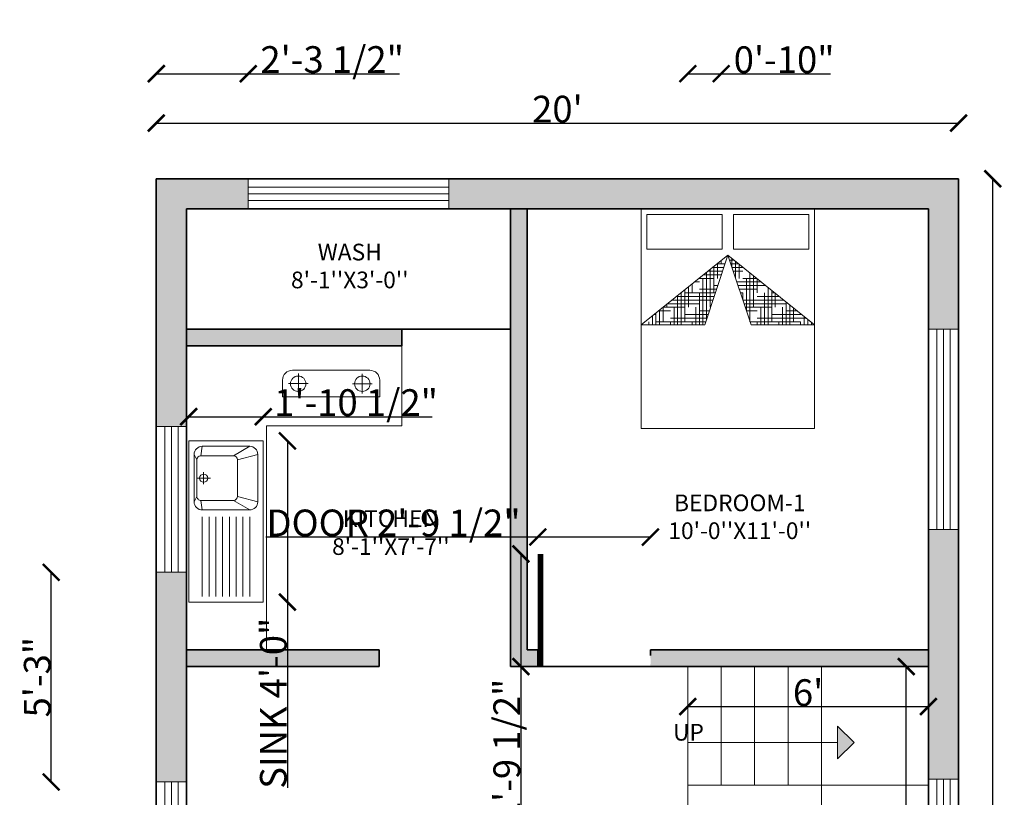
# Model space of a CAD drawing. Units: inches. Extents: x 2267 to 2908, y 1531 to 2136.
# Tile 3 of 5: x 2267 to 2562, y 1882 to 2115. Entities that reach past the tile are written whole.
import ezdxf

# ---------------------------------------------------------------- set-up
doc = ezdxf.new("R2010")
doc.units = ezdxf.units.IN
for name, color, linetype, lineweight in [('A-ANNO-DIMS', 2, 'Continuous', 18), ('A-ANNO-SYMB', 50, 'Continuous', 18), ('A-ANNO-TEXT', 7, 'Continuous', 18), ('A-AREA-IDEN', 7, 'Continuous', 18), ('A-EQPM', 9, 'Continuous', 18), ('A-FLOR-FIXT', 9, 'Continuous', 18), ('A-FURN', 9, 'Continuous', 18), ('A-WALL-PATT', 8, 'Continuous', 13), ('DOOR', 30, 'Continuous', 18), ('KITCHEN', 80, 'Continuous', 18), ('STEPS', 50, 'Continuous', 18), ('WALL', 7, 'Continuous', 35), ('WINDOW', 152, 'Continuous', 18)]:
    doc.layers.add(name, color=color, linetype=linetype, lineweight=lineweight)
doc.styles.get("Standard").update_dxf_attribs({"font": 'arial.ttf'})
doc.dimstyles.get("Standard").update_dxf_attribs({"dimtxt": 8, "dimasz": 5, "dimexe": 0.18, "dimexo": 0.0625, "dimgap": 0.09, "dimtad": 1, "dimdec": 1, "dimzin": 0, "dimdsep": 46, "dimlunit": 4, "dimtxsty": 'Standard', "dimblk": 'ARCHTICK', "dimcen": 0.09, "dimse1": 1, "dimse2": 1, "dimadec": 0, "dimazin": 0, "dimtfac": 1, "dimtdec": 1, "dimtofl": 0, "dimtmove": 0, "dimatfit": 3, "dimfxl": 1, "dimtolj": 1, "dimtzin": 0, "dimarcsym": 0})

# ---------------------------------------------------------------- blocks, each defined once
blk = doc.blocks.new('A$C73484D89')
at = {"layer": 'DOOR'}
blk.add_lwpolyline([(1, 0, 0, 0, 0), (1, 0, 0, 0, 0), (0.975, 0, 0.05, 0.05, 0), (0.975, -1, 0, 0, 0), (0.95, -1, 0, 0, -0.429311), (0, 0, 0, 0, 0), (0, 0, 0, 0, 0)], format="xyseb", dxfattribs=at)
blk = doc.blocks.new('KK')
for p, q in [((0, 0.55), (0, 0)), ((1.19, 0.55), (0, 0.55)), ((0.1, 0.51), (0.14, 0.36)), ((0.45, 0.51), (0.1, 0.51)), ((0.41, 0.36), (0.45, 0.51)), ((1.19, 0), (1.19, 0.55)), ((0.11, 0.33), (0.04, 0.45)), ((0.04, 0.45), (0.04, 0.1)), ((0.44, 0.33), (0.51, 0.45)), ((0.51, 0.1), (0.51, 0.45)), ((0.56, 0.45), (1.15, 0.45)), ((0.56, 0.4), (1.15, 0.4)), ((0.11, 0.09), (0.11, 0.33)), ((0.14, 0.36), (0.41, 0.36)), ((0.44, 0.33), (0.44, 0.09)), ((0.56, 0.35), (1.15, 0.35)), ((0.56, 0.3), (1.15, 0.3)), ((0.56, 0.25), (1.15, 0.25)), ((0.275, 0.06), (0.275, 0.16)), ((0.56, 0.2), (1.15, 0.2)), ((0.56, 0.15), (1.15, 0.15)), ((0.04, 0.1), (0.11, 0.09)), ((0.23, 0.11), (0.32, 0.11)), ((0.44, 0.09), (0.51, 0.1)), ((0.56, 0.1), (1.15, 0.1)), ((0, 0), (1.19, 0)), ((0.14, 0.06), (0.1, 0.04)), ((0.1, 0.04), (0.45, 0.04)), ((0.41, 0.06), (0.14, 0.06)), ((0.41, 0.06), (0.45, 0.04))]:
    blk.add_line(p, q)
blk.add_circle((0.275, 0.11), 0.03)
for centre, radius, start, end in [((0.1, 0.45), 0.06, 90, 180), ((0.45, 0.45), 0.06, 0, 90), ((0.14, 0.33), 0.03, 90, 180), ((0.41, 0.33), 0.03, 0, 90), ((0.1, 0.1), 0.06, 180, 270), ((0.14, 0.09), 0.03, 180, 270), ((0.41, 0.09), 0.03, 270, 0), ((0.45, 0.1), 0.06, 270, 0)]:
    blk.add_arc(centre, radius, start, end)
blk = doc.blocks.new('*X6')
at = {"color": 0}
for p, q in [((20.25, 14.8125), (20.2772, 14.8125)), ((20.1562, 14.625), (20.1562, 14.7281)), ((20.1739, 14.75), (20.2772, 14.75)), ((20.1875, 14.75), (20.1875, 14.7669)), ((20.199, 14.7812), (20.2772, 14.7812)), ((20.25, 14.3194), (20.25, 14.75)), ((20.0938, 14.375), (20.0938, 14.6504)), ((20.0984, 14.6562), (20.125, 14.6562)), ((20.1236, 14.6875), (20.25, 14.6875)), ((20.125, 14.5), (20.125, 14.6893)), ((20.1487, 14.7188), (20.2772, 14.7188)), ((20.023, 14.5625), (20.2772, 14.5625)), ((20.0312, 14.2469), (20.0312, 14.5727)), ((20.0625, 14.2573), (20.0625, 14.6116)), ((20.125, 14.5938), (20.2772, 14.5938)), ((20.2188, 14.3091), (20.2188, 14.625)), ((20.25, 14.625), (20.2772, 14.625)), ((19.9476, 14.4688), (20.125, 14.4688)), ((19.9727, 14.5), (20.25, 14.5)), ((19.9979, 14.5312), (20.2772, 14.5312)), ((20, 14.2366), (20, 14.5)), ((20.1875, 14.2987), (20.1875, 14.5)), ((19.9062, 14.375), (19.9062, 14.4174)), ((19.9225, 14.4375), (20, 14.4375)), ((20.125, 14.4062), (20.2772, 14.4062)), ((20.25, 14.4375), (20.2772, 14.4375)), ((19.8125, 14.1744), (19.8125, 14.3008)), ((19.8219, 14.3125), (20.2291, 14.3125)), ((19.8438, 14.1848), (19.8438, 14.3397)), ((19.875, 14.25), (19.875, 14.3785)), ((19.875, 14.3438), (20.2772, 14.3438)), ((19.9688, 14.2262), (19.9688, 14.375)), ((20, 14.375), (20.2772, 14.375)), ((20.1562, 14.2884), (20.1562, 14.375)), ((19.7465, 14.2188), (19.875, 14.2188)), ((19.75, 14.1537), (19.75, 14.2231)), ((19.7716, 14.25), (20, 14.25)), ((19.7812, 14.1641), (19.7812, 14.262)), ((19.7967, 14.2812), (20.125, 14.2812)), ((19.9375, 14.2159), (19.9375, 14.25)), ((19.7213, 14.1875), (19.75, 14.1875)), ((19.7018, 14.0938), (19.7786, 14.0938)), ((19.7188, 14.0726), (19.7188, 14.1136)), ((19.7269, 14.0625), (19.8728, 14.0625)), ((19.75, 14.0338), (19.75, 14.1032)), ((19.7812, 13.9949), (19.7812, 14.0929)), ((19.8125, 14), (19.8125, 14.0825)), ((19.9062, 13.8396), (19.9062, 14.0514)), ((19.9375, 13.8007), (19.9375, 14.0411)), ((19.752, 14.0312), (19.875, 14.0312)), ((19.875, 13.8784), (19.875, 14)), ((19.875, 13.9688), (20.1557, 13.9688)), ((19.9688, 13.875), (19.9688, 14.0307)), ((20, 14), (20, 14.0204)), ((20, 14), (20.0614, 14)), ((20.0625, 13.6454), (20.0625, 13.9996)), ((20.0938, 13.625), (20.0938, 13.9893)), ((20.125, 13.75), (20.125, 13.9789)), ((20.1562, 13.875), (20.1562, 13.9686)), ((19.8275, 13.9375), (20.25, 13.9375)), ((19.8526, 13.9062), (20.125, 13.9062)), ((19.8777, 13.875), (20, 13.875)), ((20.0312, 13.6842), (20.0312, 13.875)), ((20.2188, 13.4511), (20.2188, 13.875)), ((20.25, 13.5), (20.25, 13.9375)), ((20.25, 13.875), (20.2772, 13.875)), ((20, 13.8125), (20.2772, 13.8125)), ((20.125, 13.8438), (20.2772, 13.8438)), ((19.9532, 13.7812), (20.2772, 13.7812)), ((19.9783, 13.75), (20.25, 13.75)), ((20, 13.723), (20, 13.75)), ((20.0035, 13.7188), (20.125, 13.7188)), ((20.1875, 13.49), (20.1875, 13.75)), ((20.0789, 13.625), (20.2772, 13.625)), ((20.125, 13.6562), (20.2772, 13.6562)), ((20.1562, 13.5288), (20.1562, 13.625)), ((20.25, 13.6875), (20.2772, 13.6875)), ((20.104, 13.5938), (20.2772, 13.5938)), ((20.1292, 13.5625), (20.25, 13.5625)), ((20.2046, 13.4688), (20.2772, 13.4688)), ((20.25, 13.5), (20.2772, 13.5)), ((20.2297, 13.4375), (20.2772, 13.4375)), ((20.2549, 13.4062), (20.2772, 13.4062))]:
    blk.add_line(p, q, dxfattribs=at)
blk = doc.blocks.new('MAT-P13')
for p, q in [((-0.75, 0), (0.75, 0)), ((-0.75, 0), (-0.75, -1.9)), ((0.75, 0), (0.75, -1.9)), ((-0.7, -0.05), (-0.7, -0.35)), ((-0.7, -0.05), (-0.05, -0.05)), ((-0.05, -0.35), (-0.05, -0.05)), ((0.05, -0.05), (0.7, -0.05)), ((0.05, -0.35), (0.05, -0.05)), ((0.7, -0.05), (0.7, -0.35)), ((-0.75, -1.0034), (0, -0.4)), ((0, -0.4), (-0.75, -1.0034)), ((-0.7, -0.35), (-0.05, -0.35)), ((0, -0.4), (-0.2, -1.0034)), ((0, -0.4), (0.2, -1.0034)), ((0, -0.4), (0.75, -1.0034)), ((0.05, -0.35), (0.7, -0.35)), ((-0.75, -1.0034), (-0.2, -1.0034)), ((0.2, -1.0034), (0.75, -1.0034)), ((0.75, -1.9), (-0.75, -1.9))]:
    blk.add_line(p, q)
at = {"xscale": -1, "rotation": 90}
blk.add_blockref('*X6', (14.1285, 19.2738), dxfattribs=at)
blk = doc.blocks.new('_ArchTick')
at = {"color": 0, "linetype": 'ByBlock', "const_width": 0.15}
blk.add_lwpolyline([(-0.5, -0.5), (0.5, 0.5)], dxfattribs=at)
blk = doc.blocks.new('*D9')
at = {"layer": 'A-ANNO-DIMS', "color": 0, "lineweight": -2, "transparency": 16777216}
blk.add_line((2307.81, 2083.8), (2547.81, 2083.8), dxfattribs=at)
at = {"layer": 'Defpoints', "color": 0, "transparency": 16777216}
for p in [(2547.81, 2083.8), (2307.81, 2067.14), (2547.81, 2067.14)]:
    blk.add_point(p, dxfattribs=at)
at = {"layer": 'A-ANNO-DIMS', "color": 0, "lineweight": -2, "transparency": 16777216, "xscale": 5, "yscale": 5, "zscale": 5, "rotation": 180}
blk.add_blockref('_ArchTick', (2307.81, 2083.8), dxfattribs=at)
at = {"layer": 'A-ANNO-DIMS', "color": 0, "lineweight": -2, "transparency": 16777216, "xscale": 5, "yscale": 5, "zscale": 5}
blk.add_blockref('_ArchTick', (2547.81, 2083.8), dxfattribs=at)
at = {"layer": 'A-ANNO-DIMS', "color": 0, "transparency": 16777216, "insert": (2427.81, 2087.98), "char_height": 8, "attachment_point": 5}
blk.add_mtext("\\A1;20'", dxfattribs=at)
blk = doc.blocks.new('*D10')
at = {"layer": 'A-ANNO-DIMS', "color": 0, "lineweight": -2, "transparency": 16777216}
blk.add_line((2558.03, 2067.14), (2558.03, 1587.14), dxfattribs=at)
at = {"layer": 'Defpoints', "color": 0, "transparency": 16777216}
for p in [(2547.81, 2067.14), (2547.81, 1587.14), (2558.03, 1587.14)]:
    blk.add_point(p, dxfattribs=at)
at = {"layer": 'A-ANNO-DIMS', "color": 0, "lineweight": -2, "transparency": 16777216, "xscale": 5, "yscale": 5, "zscale": 5}
for p, rotation in [((2558.03, 2067.14), 90), ((2558.03, 1587.14), 270)]:
    blk.add_blockref('_ArchTick', p, dxfattribs=dict(at, rotation=rotation))
at = {"layer": 'A-ANNO-DIMS', "color": 0, "transparency": 16777216, "insert": (2553.86, 1827.14), "char_height": 8, "attachment_point": 5, "rotation": 90}
blk.add_mtext("\\A1;40'", dxfattribs=at)
blk = doc.blocks.new('*D17')
at = {"layer": 'A-ANNO-DIMS', "color": 0, "lineweight": -2, "transparency": 16777216}
blk.add_line((2532.17, 1810.14), (2532.17, 1921.14), dxfattribs=at)
at = {"layer": 'Defpoints', "color": 0, "transparency": 16777216}
for p in [(2532.17, 1921.14), (2538.81, 1921.14), (2538.81, 1810.14)]:
    blk.add_point(p, dxfattribs=at)
at = {"layer": 'A-ANNO-DIMS', "color": 0, "lineweight": -2, "transparency": 16777216, "xscale": 5, "yscale": 5, "zscale": 5}
for p, rotation in [((2532.17, 1921.14), 90), ((2532.17, 1810.14), 270)]:
    blk.add_blockref('_ArchTick', p, dxfattribs=dict(at, rotation=rotation))
at = {"layer": 'A-ANNO-DIMS', "color": 0, "transparency": 16777216, "insert": (2527.99, 1865.64), "char_height": 8, "attachment_point": 5, "rotation": 90}
blk.add_mtext('\\A1;9\'-3"', dxfattribs=at)
blk = doc.blocks.new('*D18')
at = {"layer": 'A-ANNO-DIMS', "color": 0, "lineweight": -2, "transparency": 16777216}
blk.add_line((2466.81, 1909.16), (2538.81, 1909.16), dxfattribs=at)
at = {"layer": 'Defpoints', "color": 0, "transparency": 16777216}
for p in [(2466.81, 1921.14), (2538.81, 1921.14), (2538.81, 1909.16)]:
    blk.add_point(p, dxfattribs=at)
at = {"layer": 'A-ANNO-DIMS', "color": 0, "lineweight": -2, "transparency": 16777216, "xscale": 5, "yscale": 5, "zscale": 5, "rotation": 180}
blk.add_blockref('_ArchTick', (2466.81, 1909.16), dxfattribs=at)
at = {"layer": 'A-ANNO-DIMS', "color": 0, "lineweight": -2, "transparency": 16777216, "xscale": 5, "yscale": 5, "zscale": 5}
blk.add_blockref('_ArchTick', (2538.81, 1909.16), dxfattribs=at)
at = {"layer": 'A-ANNO-DIMS', "color": 0, "transparency": 16777216, "insert": (2502.81, 1913.33), "char_height": 8, "attachment_point": 5}
blk.add_mtext("\\A1;6'", dxfattribs=at)
blk = doc.blocks.new('WIN-60IN')
for p, q in [((0, 6.5), (60, 6.5)), ((0, 4.5), (60, 4.5)), ((0, 2.5), (60, 2.5))]:
    blk.add_line(p, q)
blk.add_lwpolyline([(0, 9), (60, 9), (60, 0), (0, 0)], close=True)
blk = doc.blocks.new('WIN-43_65IN')
for p, q in [((2.5, 0), (2.5, 43.65)), ((4.5, 0), (4.5, 43.65)), ((6.5, 0), (6.5, 43.65))]:
    blk.add_line(p, q)
blk.add_lwpolyline([(0, 0), (0, 43.65), (9, 43.65), (9, 0)], close=True)
blk = doc.blocks.new('STAIR-DIRECTION-ARROW')
at = {"transparency": 33554585}
h = blk.add_hatch(color=256, dxfattribs=at)
h.dxf.hatch_style = 1
h.paths.add_polyline_path([(44.76, 9.76), (44.76, 0), (49.76, 4.88)])
for p, q in [((44.76, 9.76), (44.76, 0)), ((49.76, 4.88), (44.76, 9.76)), ((0, 4.88), (44.76, 4.88)), ((49.76, 4.88), (44.76, 0))]:
    blk.add_line(p, q)
blk = doc.blocks.new('*D31')
at = {"layer": 'A-ANNO-DIMS', "color": 0, "lineweight": -2, "transparency": 16777216}
for p, q in [((2421.94, 1959.89), (2340.62, 1959.89)), ((2455.64, 1959.89), (2421.94, 1959.89))]:
    blk.add_line(p, q, dxfattribs=at)
at = {"layer": 'Defpoints', "color": 0, "transparency": 16777216}
for p in [(2421.94, 1959.89), (2421.94, 1954.84), (2455.64, 1954.84)]:
    blk.add_point(p, dxfattribs=at)
at = {"layer": 'A-ANNO-DIMS', "color": 0, "lineweight": -2, "transparency": 16777216, "xscale": 5, "yscale": 5, "zscale": 5, "rotation": 180}
blk.add_blockref('_ArchTick', (2421.94, 1959.89), dxfattribs=at)
at = {"layer": 'A-ANNO-DIMS', "color": 0, "lineweight": -2, "transparency": 16777216, "xscale": 5, "yscale": 5, "zscale": 5}
blk.add_blockref('_ArchTick', (2455.64, 1959.89), dxfattribs=at)
at = {"layer": 'A-ANNO-DIMS', "color": 0, "transparency": 16777216, "insert": (2378.78, 1964.12), "char_height": 8, "attachment_point": 5}
blk.add_mtext('\\A1;DOOR 2\'-9 1/2"', dxfattribs=at)
blk = doc.blocks.new('*D32')
at = {"layer": 'A-ANNO-DIMS', "color": 0, "lineweight": -2, "transparency": 16777216}
for p, q in [((2416.88, 1954.84), (2416.88, 1921.14)), ((2416.88, 1921.14), (2416.88, 1875.92))]:
    blk.add_line(p, q, dxfattribs=at)
at = {"layer": 'Defpoints', "color": 0, "transparency": 16777216}
for p in [(2421.94, 1954.84), (2416.88, 1921.14), (2421.94, 1921.14)]:
    blk.add_point(p, dxfattribs=at)
at = {"layer": 'A-ANNO-DIMS', "color": 0, "lineweight": -2, "transparency": 16777216, "xscale": 5, "yscale": 5, "zscale": 5}
for p, rotation in [((2416.88, 1954.84), 90), ((2416.88, 1921.14), 270)]:
    blk.add_blockref('_ArchTick', p, dxfattribs=dict(at, rotation=rotation))
at = {"layer": 'A-ANNO-DIMS', "color": 0, "transparency": 16777216, "insert": (2412.66, 1896.03), "char_height": 8, "attachment_point": 5, "rotation": 90}
blk.add_mtext('\\A1;2\'-9 1/2"', dxfattribs=at)
blk = doc.blocks.new('*D51')
at = {"layer": 'A-ANNO-DIMS', "color": 0, "lineweight": -2, "transparency": 16777216}
for p, q in [((2347.03, 1988.68), (2347.03, 1940.44)), ((2347.03, 1940.44), (2347.03, 1884.85))]:
    blk.add_line(p, q, dxfattribs=at)
at = {"layer": 'Defpoints', "color": 0, "transparency": 16777216}
for p in [(2339.8, 1988.68), (2339.8, 1940.44), (2347.03, 1940.44)]:
    blk.add_point(p, dxfattribs=at)
at = {"layer": 'A-ANNO-DIMS', "color": 0, "lineweight": -2, "transparency": 16777216, "xscale": 5, "yscale": 5, "zscale": 5}
for p, rotation in [((2347.03, 1988.68), 90), ((2347.03, 1940.44), 270)]:
    blk.add_blockref('_ArchTick', p, dxfattribs=dict(at, rotation=rotation))
at = {"layer": 'A-ANNO-DIMS', "color": 0, "transparency": 16777216, "insert": (2342.81, 1910.15), "char_height": 8, "attachment_point": 5, "rotation": 90}
blk.add_mtext('\\A1;SINK 4\'-0"', dxfattribs=at)
blk = doc.blocks.new('*D52')
at = {"layer": 'A-ANNO-DIMS', "color": 0, "lineweight": -2, "transparency": 16777216}
for p, q in [((2317.5, 1995.92), (2339.8, 1995.92)), ((2339.8, 1995.92), (2390.35, 1995.92))]:
    blk.add_line(p, q, dxfattribs=at)
at = {"layer": 'Defpoints', "color": 0, "transparency": 16777216}
for p in [(2339.8, 1995.92), (2317.5, 1988.68), (2339.8, 1988.68)]:
    blk.add_point(p, dxfattribs=at)
at = {"layer": 'A-ANNO-DIMS', "color": 0, "lineweight": -2, "transparency": 16777216, "xscale": 5, "yscale": 5, "zscale": 5, "rotation": 180}
blk.add_blockref('_ArchTick', (2317.5, 1995.92), dxfattribs=at)
at = {"layer": 'A-ANNO-DIMS', "color": 0, "lineweight": -2, "transparency": 16777216, "xscale": 5, "yscale": 5, "zscale": 5}
blk.add_blockref('_ArchTick', (2339.8, 1995.92), dxfattribs=at)
at = {"layer": 'A-ANNO-DIMS', "color": 0, "transparency": 16777216, "insert": (2367.57, 2000.14), "char_height": 8, "attachment_point": 5}
blk.add_mtext('\\A1;1\'-10 1/2"', dxfattribs=at)
blk = doc.blocks.new('*D57')
at = {"layer": 'A-ANNO-DIMS', "color": 0, "lineweight": -2, "transparency": 16777216}
blk.add_line((2276.36, 1886.58), (2276.36, 1949.34), dxfattribs=at)
at = {"layer": 'Defpoints', "color": 0, "transparency": 16777216}
for p in [(2276.36, 1949.34), (2307.81, 1949.34), (2307.81, 1886.58)]:
    blk.add_point(p, dxfattribs=at)
at = {"layer": 'A-ANNO-DIMS', "color": 0, "lineweight": -2, "transparency": 16777216, "xscale": 5, "yscale": 5, "zscale": 5}
for p, rotation in [((2276.36, 1949.34), 90), ((2276.36, 1886.58), 270)]:
    blk.add_blockref('_ArchTick', p, dxfattribs=dict(at, rotation=rotation))
at = {"layer": 'A-ANNO-DIMS', "color": 0, "transparency": 16777216, "insert": (2272.18, 1917.96), "char_height": 8, "attachment_point": 5, "rotation": 90}
blk.add_mtext('\\A1;5\'-3"', dxfattribs=at)
blk = doc.blocks.new('*D60')
at = {"layer": 'A-ANNO-DIMS', "color": 0, "lineweight": -2, "transparency": 16777216}
for p, q in [((2307.81, 2098.59), (2335.31, 2098.59)), ((2335.31, 2098.59), (2380.53, 2098.59))]:
    blk.add_line(p, q, dxfattribs=at)
at = {"layer": 'Defpoints', "color": 0, "transparency": 16777216}
for p in [(2335.31, 2098.59), (2307.81, 2067.14), (2335.31, 2067.14)]:
    blk.add_point(p, dxfattribs=at)
at = {"layer": 'A-ANNO-DIMS', "color": 0, "lineweight": -2, "transparency": 16777216, "xscale": 5, "yscale": 5, "zscale": 5, "rotation": 180}
blk.add_blockref('_ArchTick', (2307.81, 2098.59), dxfattribs=at)
at = {"layer": 'A-ANNO-DIMS', "color": 0, "lineweight": -2, "transparency": 16777216, "xscale": 5, "yscale": 5, "zscale": 5}
blk.add_blockref('_ArchTick', (2335.31, 2098.59), dxfattribs=at)
at = {"layer": 'A-ANNO-DIMS', "color": 0, "transparency": 16777216, "insert": (2360.42, 2102.82), "char_height": 8, "attachment_point": 5}
blk.add_mtext('\\A1;2\'-3 1/2"', dxfattribs=at)
blk = doc.blocks.new('*D62')
at = {"layer": 'A-ANNO-DIMS', "color": 0, "lineweight": -2, "transparency": 16777216}
blk.add_line((2900.68, 2022.14), (2900.68, 2067.14), dxfattribs=at)
at = {"layer": 'Defpoints', "color": 0, "transparency": 16777216}
for p in [(2547.81, 2067.14), (2900.68, 2067.14), (2547.81, 2022.14)]:
    blk.add_point(p, dxfattribs=at)
at = {"layer": 'A-ANNO-DIMS', "color": 0, "lineweight": -2, "transparency": 16777216, "xscale": 5, "yscale": 5, "zscale": 5}
for p, rotation in [((2900.68, 2067.14), 90), ((2900.68, 2022.14), 270)]:
    blk.add_blockref('_ArchTick', p, dxfattribs=dict(at, rotation=rotation))
at = {"layer": 'A-ANNO-DIMS', "color": 0, "transparency": 16777216, "insert": (2896.5, 2044.64), "char_height": 8, "attachment_point": 5, "rotation": 90}
blk.add_mtext('\\A1;3\'-9"', dxfattribs=at)
blk = doc.blocks.new('*D64')
at = {"layer": 'A-ANNO-DIMS', "color": 0, "lineweight": -2, "transparency": 16777216}
for p, q in [((2466.81, 2098.59), (2476.81, 2098.59)), ((2476.81, 2098.59), (2509.47, 2098.59))]:
    blk.add_line(p, q, dxfattribs=at)
at = {"layer": 'Defpoints', "color": 0, "transparency": 16777216}
for p in [(2476.81, 2098.59), (2466.81, 1885.64), (2476.81, 1885.64)]:
    blk.add_point(p, dxfattribs=at)
at = {"layer": 'A-ANNO-DIMS', "color": 0, "lineweight": -2, "transparency": 16777216, "xscale": 5, "yscale": 5, "zscale": 5, "rotation": 180}
blk.add_blockref('_ArchTick', (2466.81, 2098.59), dxfattribs=at)
at = {"layer": 'A-ANNO-DIMS', "color": 0, "lineweight": -2, "transparency": 16777216, "xscale": 5, "yscale": 5, "zscale": 5}
blk.add_blockref('_ArchTick', (2476.81, 2098.59), dxfattribs=at)
at = {"layer": 'A-ANNO-DIMS', "color": 0, "transparency": 16777216, "insert": (2495.64, 2102.77), "char_height": 8, "attachment_point": 5}
blk.add_mtext('\\A1;0\'-10"', dxfattribs=at)
blk = doc.blocks.new('*D65')
at = {"layer": 'A-ANNO-DIMS', "color": 0, "lineweight": -2, "transparency": 16777216}
blk.add_line((2900.68, 1887.47), (2900.68, 1962.14), dxfattribs=at)
at = {"layer": 'Defpoints', "color": 0, "transparency": 16777216}
for p in [(2547.81, 1962.14), (2900.68, 1962.14), (2547.81, 1887.47)]:
    blk.add_point(p, dxfattribs=at)
at = {"layer": 'A-ANNO-DIMS', "color": 0, "lineweight": -2, "transparency": 16777216, "xscale": 5, "yscale": 5, "zscale": 5}
for p, rotation in [((2900.68, 1962.14), 90), ((2900.68, 1887.47), 270)]:
    blk.add_blockref('_ArchTick', p, dxfattribs=dict(at, rotation=rotation))
at = {"layer": 'A-ANNO-DIMS', "color": 0, "transparency": 16777216, "insert": (2896.45, 1924.8), "char_height": 8, "attachment_point": 5, "rotation": 90}
blk.add_mtext('\\A1;6\'-2 1/2"', dxfattribs=at)

msp = doc.modelspace()

# ---------------------------------------------------------------- hatches: boundary and pattern name
at = {"layer": 'A-WALL-PATT', "transparency": 33554585}
h = msp.add_hatch(color=256, dxfattribs=at)
h.dxf.hatch_style = 1
h.paths.add_polyline_path([(2547.81, 2067.14), (2395.31, 2067.14), (2395.31, 2058.14), (2413.81, 2058.14), (2538.81, 2058.14), (2538.81, 2022.14), (2547.81, 2022.14)])
h.paths.add_polyline_path([(2335.31, 2067.14), (2307.81, 2067.14), (2307.81, 1992.99), (2316.81, 1992.99), (2316.81, 2058.14), (2335.31, 2058.14)])
h.paths.add_polyline_path([(2316.81, 1949.34), (2307.81, 1949.34), (2307.81, 1886.58), (2316.81, 1886.58)])
h.paths.add_polyline_path([(2316.81, 1842.93), (2307.81, 1842.93), (2307.81, 1791.76), (2316.81, 1791.76)])
h.paths.add_polyline_path([(2316.81, 1769.93), (2307.81, 1769.93), (2307.81, 1695.97), (2316.81, 1695.97)])
h.paths.add_polyline_path([(2316.81, 1652.32), (2307.81, 1652.32), (2307.81, 1587.14), (2344.81, 1587.14), (2344.81, 1596.14), (2316.81, 1596.14)])
h.paths.add_polyline_path([(2441.81, 1715.23, -0.025641), (2438.4, 1715.23), (2436.81, 1715.23), (2436.81, 1596.14), (2404.81, 1596.14), (2404.81, 1587.14), (2441.81, 1587.14)])
h.paths.add_polyline_path([(2547.81, 1770.23), (2538.81, 1770.23), (2538.81, 1752.14), (2542.81, 1752.14), (2542.81, 1587.14), (2547.81, 1587.14)])
h.paths.add_polyline_path([(2547.81, 1843.82), (2538.81, 1843.82), (2538.81, 1792.05), (2547.81, 1792.05)])
h.paths.add_polyline_path([(2547.81, 1962.14), (2538.81, 1962.14), (2538.81, 1887.47), (2547.81, 1887.47)])
h.paths.add_polyline_path([(2638.23, 1962.08), (2629.23, 1962.08), (2629.23, 1885.88), (2638.23, 1885.88)])
h.paths.add_polyline_path([(2638.23, 2056.17), (2860.23, 2056.17), (2860.23, 2020.17), (2869.23, 2020.17), (2869.23, 2065.17), (2629.23, 2065.17), (2629.23, 2022.08), (2638.23, 2022.08)])
h.paths.add_polyline_path([(2869.23, 1960.17), (2860.23, 1960.17), (2860.23, 1885.5), (2869.23, 1885.5)])
h.paths.add_polyline_path([(2869.23, 1841.85), (2860.23, 1841.85), (2860.23, 1790.08), (2869.23, 1790.08)])
h.paths.add_polyline_path([(2869.23, 1768.26), (2860.23, 1768.26), (2860.23, 1768.05), (2860.23, 1720.44), (2869.23, 1720.44)])
h.paths.add_polyline_path([(2869.23, 1660.44), (2860.23, 1660.44), (2860.23, 1585.17), (2869.23, 1585.17)])
h.paths.add_polyline_path([(2763.23, 1594.17), (2726.23, 1594.17), (2726.23, 1585.17), (2763.23, 1585.17)])
h.paths.add_polyline_path([(2666.23, 1594.17), (2638.23, 1594.17), (2638.23, 1768.3), (2629.23, 1768.3), (2629.23, 1585.17), (2666.23, 1585.17)])
h.paths.add_polyline_path([(2638.23, 1842.24), (2629.23, 1842.24), (2629.23, 1790.12), (2638.23, 1790.12)])
h = msp.add_hatch(color=256, dxfattribs=at)
h.dxf.hatch_style = 1
h.paths.add_polyline_path([(2763.23, 1755.17), (2758.23, 1755.17), (2758.23, 1625.17), (2760.21, 1625.17, -0.025641), (2763.23, 1625.17)])
h.paths.add_polyline_path([(2638.23, 1750.17), (2679.86, 1750.17, -0.025641), (2679.86, 1752.99), (2679.86, 1755.17), (2638.23, 1755.17)])
h.paths.add_polyline_path([(2860.23, 1625.17), (2860.23, 1630.17), (2796.25, 1630.17), (2796.25, 1628.39, -0.025641), (2796.25, 1625.17)])
h.paths.add_polyline_path([(2730.26, 1919.17), (2745.45, 1919.17), (2745.45, 1924.17), (2740.23, 1924.17), (2740.23, 2056.17), (2735.23, 2056.17), (2735.23, 1924.17), (2730.26, 1924.17)])
h.paths.add_polyline_path([(2860.23, 1919.17), (2860.23, 1924.17), (2774.38, 1924.17), (2774.38, 1921.99, -0.025641), (2774.38, 1919.17)])
h.paths.add_polyline_path([(2638.23, 1919.17), (2701.33, 1919.17, -0.025641), (2701.33, 1921.99), (2701.33, 1924.17), (2638.23, 1924.17)])
h.paths.add_polyline_path([(2538.81, 1752.14), (2538.81, 1757.14), (2441.81, 1757.14), (2441.81, 1762.09), (2439.73, 1762.09, -0.025641), (2436.81, 1762.09), (2436.81, 1750.17), (2441.81, 1750.17), (2441.81, 1752.14)])
h.paths.add_polyline_path([(2436.81, 1810.14), (2436.81, 1792.08), (2441.81, 1792.08), (2441.81, 1805.14), (2538.81, 1805.14), (2538.81, 1810.14)])
h.paths.add_polyline_path([(2346.81, 1805.14), (2346.81, 1810.14), (2316.81, 1810.14), (2316.81, 1805.14)], flags=0)
h.paths.add_polyline_path([(2376.81, 1810.14), (2371.81, 1810.14), (2371.81, 1757.14), (2316.81, 1757.14), (2316.81, 1752.14), (2376.81, 1752.14)])
h.paths.add_polyline_path([(2374.47, 1921.14), (2374.47, 1926.14), (2316.81, 1926.14), (2316.81, 1921.14)])
h.paths.add_polyline_path([(2413.81, 1921.14), (2421.94, 1921.14), (2421.94, 1926.14), (2418.81, 1926.14), (2418.81, 2058.14), (2413.81, 2058.14)])
h.paths.add_polyline_path([(2316.81, 2022.14), (2316.81, 2017.14), (2381.27, 2017.14), (2381.27, 2022.14)])
h.paths.add_polyline_path([(2455.63, 1926.14), (2455.63, 1924.43, -0.025641), (2455.63, 1921.14), (2538.81, 1921.14), (2538.81, 1926.14)])

# ---------------------------------------------------------------- linework, layer by layer
at = {"layer": 'A-EQPM'}
for p, q in [((2348.56, 2009.83), (2371.66, 2009.83)), ((2345.56, 2001.86), (2345.56, 2006.83)), ((2350.32, 2002.97), (2350.32, 2008.8)), ((2369.43, 2002.87), (2369.43, 2008.7)), ((2374.66, 2001.86), (2374.66, 2006.83)), ((2347.4, 2005.88), (2353.23, 2005.88)), ((2366.52, 2005.78), (2372.35, 2005.78)), ((2345.56, 2001.86), (2374.66, 2001.86))]:
    msp.add_line(p, q, dxfattribs=at)
for centre in [(2350.26, 2005.78), (2369.43, 2005.78)]:
    msp.add_circle(centre, 2.31, dxfattribs=at)
for centre, start, end in [((2348.56, 2006.83), 90, 180), ((2371.66, 2006.83), 0, 90)]:
    msp.add_arc(centre, 3, start, end, dxfattribs=at)
at = {"layer": 'KITCHEN'}
for p, q in [((2381.27, 1993.14), (2381.27, 2017.14)), ((2340.81, 1993.14), (2381.27, 1993.14)), ((2340.81, 1993.14), (2340.81, 1926.14))]:
    msp.add_line(p, q, dxfattribs=at)
at = {"layer": 'STEPS'}
for p, q in [((2466.81, 1921.14), (2466.81, 1875.64)), ((2476.81, 1921.14), (2476.81, 1885.64)), ((2486.81, 1921.14), (2486.81, 1885.64)), ((2496.81, 1921.14), (2496.81, 1885.64)), ((2506.81, 1921.14), (2506.81, 1845.64)), ((2466.81, 1885.64), (2538.81, 1885.64))]:
    msp.add_line(p, q, dxfattribs=at)
at = {"layer": 'WALL'}
for p, q in [((2307.81, 2067.14), (2547.81, 2067.14)), ((2307.81, 2067.14), (2307.81, 1587.14)), ((2547.81, 2067.14), (2547.81, 1587.14)), ((2316.81, 2058.14), (2413.81, 2058.14)), ((2316.81, 2058.14), (2316.81, 1596.14)), ((2413.81, 2058.14), (2413.81, 1921.14)), ((2413.81, 2058.14), (2538.81, 2058.14)), ((2418.81, 2058.14), (2418.81, 1926.14)), ((2538.81, 2058.14), (2538.81, 1752.14)), ((2316.81, 2022.14), (2413.81, 2022.14)), ((2381.27, 2022.14), (2381.27, 2017.14)), ((2316.81, 2017.14), (2381.27, 2017.14)), ((2316.81, 1926.14), (2374.47, 1926.14)), ((2374.47, 1926.14), (2374.47, 1921.14)), ((2418.81, 1926.14), (2421.94, 1926.14)), ((2421.94, 1926.14), (2421.94, 1921.14)), ((2455.63, 1926.14), (2455.63, 1924.43)), ((2455.63, 1926.14), (2538.81, 1926.14)), ((2316.81, 1921.14), (2374.47, 1921.14)), ((2413.81, 1921.14), (2538.81, 1921.14))]:
    msp.add_line(p, q, dxfattribs=at)

# ---------------------------------------------------------------- block references
at = {"layer": 'A-ANNO-SYMB'}
msp.add_blockref('STAIR-DIRECTION-ARROW', (2466.81, 1893.51), dxfattribs=at)
at = {"layer": 'A-FLOR-FIXT', "xscale": 40.53634319473337, "yscale": 40.53634319473337, "zscale": 40.53634319473337, "rotation": 270}
msp.add_blockref('KK', (2317.5, 1988.68), dxfattribs=at)
at = {"layer": 'A-FURN', "xscale": 34.62184577987068, "yscale": 34.62184577987068, "zscale": 34.62184577987068}
msp.add_blockref('MAT-P13', (2478.81, 2058.14), dxfattribs=at)
at = {"layer": 'DOOR', "xscale": 33.69300039322582, "yscale": 33.69300039322582, "zscale": 33.69300039322582, "rotation": 180}
msp.add_blockref('A$C73484D89', (2455.63, 1921.14), dxfattribs=at)
at = {"layer": 'WINDOW'}
for name, p in [('WIN-60IN', (2335.31, 2058.14)), ('WIN-43_65IN', (2307.81, 1949.34)), ('WIN-43_65IN', (2307.81, 1842.93)), ('WIN-43_65IN', (2538.81, 1843.82))]:
    msp.add_blockref(name, p, dxfattribs=at)
at = {"layer": 'WINDOW', "rotation": 89.99999999999793}
msp.add_blockref('WIN-60IN', (2547.81, 1962.14), dxfattribs=at)

# ---------------------------------------------------------------- texts
at = {"layer": 'A-ANNO-TEXT', "insert": (2446.31, 1903.97), "char_height": 5, "attachment_point": 1}
msp.add_mtext_dynamic_manual_height_columns('\\pxqc;UP', width=41.4104, gutter_width=12.5, heights=[0], dxfattribs=at)
at = {"layer": 'A-AREA-IDEN', "char_height": 5, "attachment_point": 1}
for s, insert in [("\\pxqc;WASH\\P8'-1''X3'-0''", (2344.98, 2047.69)), ("\\pxqc;BEDROOM-1\\P10'-0''X11'-0''", (2461.66, 1972.63)), ("\\pxqc;KITCHEN\\P8'-1''X7'-7''", (2357.27, 1967.89))]:
    msp.add_mtext_dynamic_manual_height_columns(s, width=41.4104, gutter_width=12.5, heights=[0], dxfattribs=dict(at, insert=insert))

# ---------------------------------------------------------------- dimensions: what is measured, and where the dimension line sits
at = {"layer": 'A-ANNO-DIMS'}
for base, p1, p2, override, picture, middle in [((2335.31, 2098.59), (2307.81, 2067.14), (2335.31, 2067.14), {"dimdec": 1, "dimlfac": 1, "dimrnd": 0, "dimzin": 1, "dimdsep": 46, "dimlunit": 4, "dimfrac": 2}, '*D60', (2360.42, 2102.82)), ((2476.81, 2098.59), (2466.81, 1885.64), (2476.81, 1885.64), {"dimdec": 1, "dimlfac": 1, "dimrnd": 0, "dimzin": 1, "dimdsep": 46, "dimlunit": 4, "dimfrac": 2}, '*D64', (2495.64, 2102.77)), ((2547.81, 2083.8), (2307.81, 2067.14), (2547.81, 2067.14), {"dimclrd": 0, "dimclre": 0, "dimclrt": 0}, '*D9', (2427.81, 2087.98)), ((2339.8, 1995.92), (2317.5, 1988.68), (2339.8, 1988.68), {"dimdec": 1, "dimlfac": 1, "dimrnd": 0, "dimzin": 1, "dimdsep": 46, "dimlunit": 4, "dimfrac": 2}, '*D52', (2367.57, 2000.14)), ((2538.81, 1909.16), (2466.81, 1921.14), (2538.81, 1921.14), {"dimclrd": 0, "dimclre": 0, "dimclrt": 0}, '*D18', (2502.81, 1913.33))]:
    dim = msp.add_linear_dim(base=base, p1=p1, p2=p2, dimstyle='Standard', override=override, dxfattribs=at)
    dim.commit()
    dim.dimension.update_dxf_attribs({"geometry": picture, "text_midpoint": middle})
for base, p1, p2, angle, override, picture, middle in [((2558.03, 1587.14), (2547.81, 2067.14), (2547.81, 1587.14), 90, {"dimclrd": 0, "dimclre": 0, "dimclrt": 0}, '*D10', (2553.86, 1827.14)), ((2900.68, 2067.14), (2547.81, 2022.14), (2547.81, 2067.14), 90, {"dimdec": 1, "dimlfac": 1, "dimrnd": 0, "dimzin": 1, "dimdsep": 46, "dimlunit": 4, "dimfrac": 2}, '*D62', (2896.5, 2044.64)), ((2900.68, 1962.14), (2547.81, 1887.47), (2547.81, 1962.14), 90, {"dimdec": 1, "dimlfac": 1, "dimrnd": 0, "dimzin": 1, "dimdsep": 46, "dimlunit": 4, "dimfrac": 2}, '*D65', (2896.45, 1924.8)), ((2416.88, 1921.14), (2421.94, 1954.84), (2421.94, 1921.14), 270, {"dimdec": 1, "dimlfac": 1, "dimrnd": 0, "dimzin": 1, "dimdsep": 46, "dimlunit": 4, "dimfrac": 2}, '*D32', (2412.66, 1896.03)), ((2276.36, 1949.34), (2307.81, 1886.58), (2307.81, 1949.34), 90, {"dimdec": 1, "dimlfac": 1, "dimrnd": 0, "dimzin": 1, "dimdsep": 46, "dimlunit": 4, "dimfrac": 2}, '*D57', (2272.18, 1917.96)), ((2532.17, 1921.14), (2538.81, 1810.14), (2538.81, 1921.14), 90, {"dimclrd": 0, "dimclre": 0, "dimclrt": 0}, '*D17', (2527.99, 1865.64))]:
    dim = msp.add_linear_dim(base=base, p1=p1, p2=p2, angle=angle, dimstyle='Standard', override=override, dxfattribs=at)
    dim.commit()
    dim.dimension.update_dxf_attribs({"geometry": picture, "text_midpoint": middle})
for base, p1, p2, angle, text, picture, middle in [((2347.03, 1940.44), (2339.8, 1988.68), (2339.8, 1940.44), 270, 'SINK <>', '*D51', (2342.81, 1910.15)), ((2421.94, 1959.89), (2455.64, 1954.84), (2421.94, 1954.84), 180, 'DOOR <>', '*D31', (2378.78, 1964.12))]:
    dim = msp.add_linear_dim(base=base, p1=p1, p2=p2, angle=angle, text=text, dimstyle='Standard', override={"dimdec": 1, "dimlfac": 1, "dimrnd": 0, "dimzin": 1, "dimdsep": 46, "dimlunit": 4, "dimfrac": 2}, dxfattribs=at)
    dim.commit()
    dim.dimension.update_dxf_attribs({"geometry": picture, "text_midpoint": middle})

doc.saveas('drawing.dxf')
